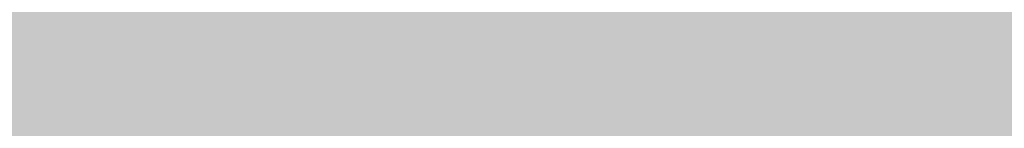
# Model space of a CAD drawing. Units: feet. Extents: x 3168 to 4724, y 827 to 1477.
# Tile 112 of 256: x 3284.48 to 3298.68, y 1096.78 to 1098.34. Entities that reach past the tile are written whole.
import ezdxf

# ---------------------------------------------------------------- set-up
doc = ezdxf.new("R2010")
doc.units = ezdxf.units.FT
doc.layers.add('A-ELEV-PATT', color=8, linetype='Continuous', lineweight=13)

msp = doc.modelspace()

# ---------------------------------------------------------------- hatches: boundary and pattern name
at = {"layer": 'A-ELEV-PATT'}
h = msp.add_hatch(color=256, dxfattribs=at)
h.dxf.hatch_style = 1
edge = h.paths.add_edge_path()
edge.add_ellipse((3552.906, 979.22), major_axis=(36.745, 0), ratio=0.484848, start_angle=0, end_angle=360)
edge = h.paths.add_edge_path()
edge.add_ellipse((3559.892, 929.252), major_axis=(36.745, 0), ratio=0.484848, start_angle=0, end_angle=360)
edge = h.paths.add_edge_path()
edge.add_line((3299.317, 1198.606), (3479.917, 1198.606))
edge.add_line((3479.917, 1198.606), (3479.917, 1209.869))
edge.add_spline(control_points=[(3479.917, 1209.869), (3464.301, 1209.869), (3448.686, 1209.869), (3410.949, 1209.869), (3388.828, 1209.869), (3355.647, 1209.869), (3344.586, 1209.869), (3327.996, 1209.869), (3322.466, 1209.869), (3314.17, 1209.869), (3311.405, 1209.869), (3307.257, 1209.869), (3305.875, 1209.869), (3303.801, 1209.869), (3303.11, 1209.869), (3302.073, 1209.869), (3301.727, 1209.869), (3301.209, 1209.869), (3301.036, 1209.869), (3300.777, 1209.869), (3300.69, 1209.869), (3300.561, 1209.869), (3300.517, 1209.869), (3300.453, 1209.869), (3300.431, 1209.869), (3300.399, 1209.869), (3300.388, 1209.869), (3300.366, 1209.869), (3300.346, 1209.869), (3300.346, 1209.869), (3300.346, 1209.869), (3300.343, 1209.869), (3300.341, 1209.869), (3300.338, 1209.869), (3300.337, 1209.869), (3300.334, 1209.869), (3300.332, 1209.869), (3300.326, 1209.869), (3300.321, 1209.869), (3300.311, 1209.869), (3300.306, 1209.869), (3300.291, 1209.869), (3300.28, 1209.869), (3300.232, 1209.869), (3300.195, 1209.869), (3299.951, 1209.871), (3299.745, 1209.874), (3299.437, 1209.883), (3299.334, 1209.887), (3299.181, 1209.893), (3299.13, 1209.895), (3298.652, 1209.917), (3298.229, 1209.946), (3297.602, 1210.002), (3297.393, 1210.023), (3297.083, 1210.058), (3296.979, 1210.07), (3296.293, 1210.155), (3295.718, 1210.243), (3294.869, 1210.399), (3294.588, 1210.454), (3294.169, 1210.543), (3294.03, 1210.574), (3291.707, 1211.101), (3289.654, 1211.813), (3285.776, 1213.564), (3283.951, 1214.603), (3280.512, 1216.98), (3278.897, 1218.318), (3276.38, 1220.829), (3275.416, 1221.918), (3274.039, 1223.708), (3273.581, 1224.35), (3273.143, 1225.016)], knot_values=[39.119033, 39.119033, 39.119033, 39.119033, 39.286353, 39.286353, 39.523379, 39.523379, 39.641892, 39.641892, 39.701148, 39.701148, 39.730777, 39.730777, 39.745591, 39.745591, 39.752998, 39.752998, 39.756701, 39.756701, 39.758553, 39.758553, 39.759479, 39.759479, 39.759942, 39.759942, 39.760173, 39.760173, 39.760289, 39.760289, 39.760405, 39.760405, 39.760463, 39.760463, 39.763389, 39.763389, 39.764851, 39.764851, 39.767304, 39.767304, 39.773825, 39.773825, 39.78057, 39.78057, 39.79477, 39.79477, 39.845194, 39.845194, 40.126715, 40.126715, 40.267476, 40.267476, 40.337856, 40.337856, 40.927023, 40.927023, 41.221606, 41.221606, 41.368898, 41.368898, 42.202622, 42.202622, 42.619485, 42.619485, 42.827916, 42.827916, 46.118323, 46.118323, 49.408731, 49.408731, 52.699139, 52.699139, 54.927489, 54.927489, 56.104228, 56.104228, 56.104228, 56.104228], weights=[1, 1, 1, 1, 1, 1, 1, 1, 1, 1, 1, 1, 1, 1, 1, 1, 1, 1, 1, 1, 1, 1, 1, 1, 1, 1, 1, 1, 1, 1, 1, 1, 1, 1, 1, 1, 1, 1, 1, 1, 1, 1, 1, 1, 1, 1, 1, 1, 1, 1, 1, 1, 1, 1, 1, 1, 1, 1, 1, 1, 1, 1, 1, 1, 1, 1, 1, 1, 1, 1, 1, 1, 1, 1], degree=3, periodic=0)
edge.add_line((3273.143, 1225.016), (3273.143, 1099.016))
edge.add_line((3273.143, 1099.016), (3299.317, 1099.016))
edge.add_line((3299.317, 1099.016), (3299.317, 1198.606))
edge = h.paths.add_edge_path()
edge.add_line((3304.758, 1324.158), (3479.917, 1324.158))
edge.add_line((3479.917, 1324.158), (3479.917, 1335.715))
edge.add_line((3479.917, 1335.715), (3269.162, 1335.715))
edge.add_spline(control_points=[(3269.162, 1335.715), (3264.024, 1335.715), (3258.364, 1328.958), (3259.264, 1323.9)], knot_values=[0, 0, 0, 0, 15.412191, 15.412191, 15.412191, 15.412191], degree=3, periodic=0)
edge.add_line((3259.264, 1323.9), (3265.517, 1288.769))
edge.add_line((3265.517, 1288.769), (3275.265, 1261.546))
edge.add_line((3275.265, 1261.546), (3304.758, 1261.546))
edge.add_line((3304.758, 1261.546), (3304.758, 1324.158))
h = msp.add_hatch(color=256, dxfattribs=at)
h.dxf.hatch_style = 1
h.paths.add_polyline_path([(3384.525, 1099.016), (3335.029, 1099.016), (3299.317, 1099.016), (3273.143, 1099.016), (3217.565, 1099.016), (3168.069, 827.116), (3335.029, 827.116)])

doc.saveas('drawing.dxf')
